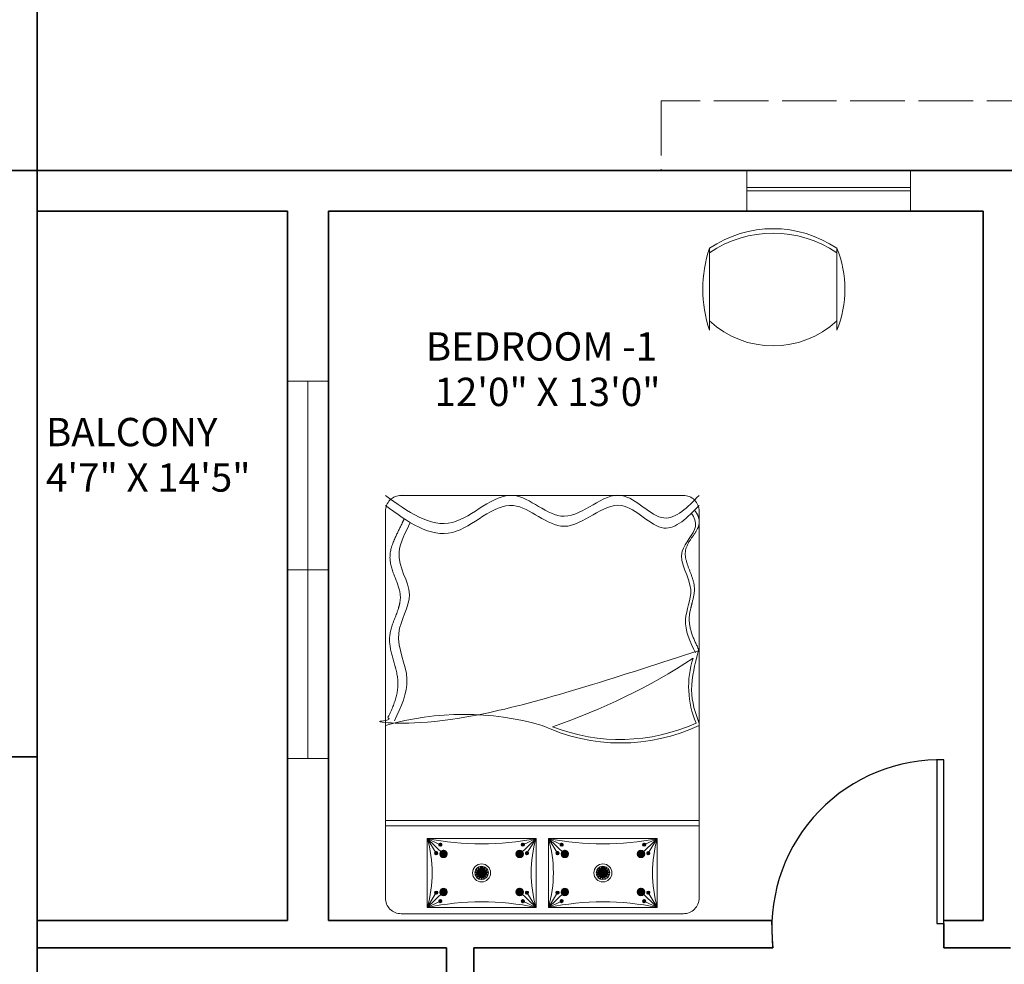
# Model space of a CAD drawing. Units: inches. Extents: x -61 to 1599, y -1316 to 257.
# Tile 166 of 204: x 998 to 1214, y -787 to -579. Entities that reach past the tile are written whole.
import ezdxf

# ---------------------------------------------------------------- set-up
doc = ezdxf.new("R2010")
doc.units = ezdxf.units.IN
doc.header["$MEASUREMENT"] = 0
doc.linetypes.add('ACAD_ISO02W100', pattern=[15, 12, -3])
for name, color, linetype, lineweight in [('A-AREA-IDEN', 1, 'Continuous', 18), ('A-FLOR-OVHD', 203, 'ACAD_ISO02W100', 13), ('A-WALL-JAMB', 4, 'ACAD_ISO02W100', 25), ('DOORS', 2, 'Continuous', 25), ('FURNITURE', 83, 'Continuous', 18), ('WALLS', 4, 'Continuous', 35), ('WINDOWS', 220, 'Continuous', 18)]:
    doc.layers.add(name, color=color, linetype=linetype, lineweight=lineweight)
doc.layers.add('LT', color=8, linetype='Continuous')
doc.styles.get("Standard").update_dxf_attribs({"font": 'arial.ttf'})

# ---------------------------------------------------------------- blocks, each defined once
blk = doc.blocks.new('DOOR-SWING-36')
blk.add_line((0, 0), (0, -5.4))
blk.add_lwpolyline([(0, 0), (0, 36), (-1.57, 36), (-1.57, 0)], close=True)
blk.add_arc((-0.74, -1.08), 37.09, 91.2913, 186.6905)
blk = doc.blocks.new('WIN-36IN')
for p, q in [((0, 4.5), (0, 9)), ((0, 9), (0, 0)), ((36, 9), (36, 0)), ((0, 5.26), (36, 5.26)), ((0, 4.5), (36, 4.5)), ((0, 4.5), (36, 4.5))]:
    blk.add_line(p, q)
blk = doc.blocks.new('WIN-83IN')
for p, q in [((0, 82.94), (9, 82.94)), ((0, 0), (9, 0))]:
    blk.add_line(p, q)
for points in [[(9, 82.94), (4.5, 82.94), (4.5, 41.47), (9, 41.47)], [(4.5, 41.47), (0, 41.47), (0, 0), (4.5, 0)]]:
    blk.add_lwpolyline(points, close=True)
blk = doc.blocks.new('BEDROOM-CHAIR')
for p, q in [((1.45, 3.47), (1.45, 21.47)), ((29.49, 3.47), (29.49, 21.47))]:
    blk.add_line(p, q)
for centre, radius, start, end in [((15.47, 0.83), 24.95, 55.8098, 124.1902), ((15.47, -0.17), 24.95, 55.8098, 124.1902), ((28.58, 12.47), 28.58, 161.6455, 198.3545), ((7.26, 12.47), 23.99, 337.9646, 22.0354), ((15.47, 20.69), 20.68, 227.332, 312.668)]:
    blk.add_arc(centre, radius, start, end)
blk = doc.blocks.new('*U15')
at = {"layer": 'LT'}
blk.add_line((0, 0.18), (0, -0.18), dxfattribs=at)
for centre, start, end in [((0.51, 0), 160.9983, 199.0017), ((-0.51, 0), 340.9983, 19.0017)]:
    blk.add_arc(centre, 0.539, start, end, dxfattribs=at)
blk = doc.blocks.new('*U16')
at = {"layer": 'LT', "transparency": 16777216}
for p, rotation in [((-66.65, -18.83), 96), ((-66.64, -18.76), 72), ((-66.63, -18.9), 120), ((-66.61, -18.69), 48.00000000000001), ((-66.58, -18.95), 144), ((-66.55, -18.65), 24), ((-66.51, -18.98), 168.0000000000001), ((-66.4, -18.65), 336.0000000000001), ((-66.37, -18.95), 216), ((-66.44, -18.98), 192), ((-66.34, -18.69), 312), ((-66.32, -18.9), 240), ((-66.31, -18.76), 288.0000000000001), ((-66.3, -18.83), 264)]:
    blk.add_blockref('*U15', p, dxfattribs=dict(at, rotation=rotation))
blk.add_blockref('*U15', (-66.48, -18.63), dxfattribs=at)
blk = doc.blocks.new('*U45')
at = {"layer": 'LT'}
blk.add_line((0, 0.18), (0, -0.18), dxfattribs=at)
for centre, start, end in [((0.51, 0), 160.9983, 199.0017), ((-0.51, 0), 340.9983, 19.0017)]:
    blk.add_arc(centre, 0.539, start, end, dxfattribs=at)
blk = doc.blocks.new('*U46')
at = {"layer": 'LT', "transparency": 16777216}
for p, rotation in [((-66.65, -18.83), 96), ((-66.64, -18.76), 72), ((-66.63, -18.9), 120), ((-66.61, -18.69), 48.00000000000001), ((-66.58, -18.95), 144), ((-66.55, -18.65), 24), ((-66.51, -18.98), 168.0000000000001), ((-66.4, -18.65), 336.0000000000001), ((-66.37, -18.95), 216), ((-66.44, -18.98), 192), ((-66.34, -18.69), 312), ((-66.32, -18.9), 240), ((-66.31, -18.76), 288.0000000000001), ((-66.3, -18.83), 264)]:
    blk.add_blockref('*U45', p, dxfattribs=dict(at, rotation=rotation))
blk.add_blockref('*U45', (-66.48, -18.63), dxfattribs=at)
blk = doc.blocks.new('*U9')
at = {"layer": 'LT'}
blk.add_line((0, 0.18), (0, -0.18), dxfattribs=at)
for centre, start, end in [((0.51, 0), 160.9983, 199.0017), ((-0.51, 0), 340.9983, 19.0017)]:
    blk.add_arc(centre, 0.539, start, end, dxfattribs=at)
blk = doc.blocks.new('*U10')
at = {"layer": 'LT', "transparency": 16777216}
for p, rotation in [((-66.65, -18.83), 96), ((-66.64, -18.76), 72), ((-66.63, -18.9), 120), ((-66.61, -18.69), 48.00000000000001), ((-66.58, -18.95), 144), ((-66.55, -18.65), 24), ((-66.51, -18.98), 168.0000000000001), ((-66.4, -18.65), 336.0000000000001), ((-66.37, -18.95), 216), ((-66.44, -18.98), 192), ((-66.34, -18.69), 312), ((-66.32, -18.9), 240), ((-66.31, -18.76), 288.0000000000001), ((-66.3, -18.83), 264)]:
    blk.add_blockref('*U9', p, dxfattribs=dict(at, rotation=rotation))
blk.add_blockref('*U9', (-66.48, -18.63), dxfattribs=at)
blk = doc.blocks.new('*U39')
at = {"layer": 'LT'}
blk.add_line((0, 0.18), (0, -0.18), dxfattribs=at)
for centre, start, end in [((0.51, 0), 160.9983, 199.0017), ((-0.51, 0), 340.9983, 19.0017)]:
    blk.add_arc(centre, 0.539, start, end, dxfattribs=at)
blk = doc.blocks.new('*U40')
at = {"layer": 'LT', "transparency": 16777216}
for p, rotation in [((-66.65, -18.83), 96), ((-66.64, -18.76), 72), ((-66.63, -18.9), 120), ((-66.61, -18.69), 48.00000000000001), ((-66.58, -18.95), 144), ((-66.55, -18.65), 24), ((-66.51, -18.98), 168.0000000000001), ((-66.4, -18.65), 336.0000000000001), ((-66.37, -18.95), 216), ((-66.44, -18.98), 192), ((-66.34, -18.69), 312), ((-66.32, -18.9), 240), ((-66.31, -18.76), 288.0000000000001), ((-66.3, -18.83), 264)]:
    blk.add_blockref('*U39', p, dxfattribs=dict(at, rotation=rotation))
blk.add_blockref('*U39', (-66.48, -18.63), dxfattribs=at)
blk = doc.blocks.new('*U17')
at = {"layer": 'LT'}
blk.add_line((0, 0.41), (0, -0.41), dxfattribs=at)
for centre, start, end in [((1.2, 0), 160.9983, 199.0017), ((-1.2, 0), 340.9983, 19.0017)]:
    blk.add_arc(centre, 1.27, start, end, dxfattribs=at)
blk = doc.blocks.new('*U18')
at = {"layer": 'LT', "transparency": 16777216}
for p, rotation in [((-156.74, -44.28), 96), ((-156.73, -44.11), 72), ((-156.69, -44.44), 120), ((-156.64, -43.96), 48.00000000000001), ((-156.58, -44.57), 144), ((-156.5, -43.86), 24), ((-156.42, -44.64), 168), ((-156.17, -43.86), 336.0000000000001), ((-156.25, -44.64), 192), ((-156.09, -44.57), 216), ((-156.03, -43.96), 312), ((-155.98, -44.44), 240), ((-155.94, -44.11), 288.0000000000001), ((-155.92, -44.28), 264)]:
    blk.add_blockref('*U17', p, dxfattribs=dict(at, rotation=rotation))
blk.add_blockref('*U17', (-156.33, -43.82), dxfattribs=at)
blk = doc.blocks.new('*U33')
at = {"layer": 'LT'}
blk.add_line((0, 0.41), (0, -0.41), dxfattribs=at)
for centre, start, end in [((1.2, 0), 160.9983, 199.0017), ((-1.2, 0), 340.9983, 19.0017)]:
    blk.add_arc(centre, 1.27, start, end, dxfattribs=at)
blk = doc.blocks.new('*U34')
at = {"layer": 'LT', "transparency": 16777216}
for p, rotation in [((-156.74, -44.28), 96), ((-156.73, -44.11), 72), ((-156.69, -44.44), 120), ((-156.64, -43.96), 48.00000000000001), ((-156.58, -44.57), 144), ((-156.5, -43.86), 24), ((-156.42, -44.64), 168), ((-156.17, -43.86), 336.0000000000001), ((-156.25, -44.64), 192), ((-156.09, -44.57), 216), ((-156.03, -43.96), 312), ((-155.98, -44.44), 240), ((-155.94, -44.11), 288.0000000000001), ((-155.92, -44.28), 264)]:
    blk.add_blockref('*U33', p, dxfattribs=dict(at, rotation=rotation))
blk.add_blockref('*U33', (-156.33, -43.82), dxfattribs=at)
blk = doc.blocks.new('*U11')
at = {"layer": 'LT'}
blk.add_line((0, 0.74), (0, -0.74), dxfattribs=at)
for centre, start, end in [((2.15, 0), 160.9983, 199.0017), ((-2.15, 0), 340.9983, 19.0017)]:
    blk.add_arc(centre, 2.27, start, end, dxfattribs=at)
blk = doc.blocks.new('*U12')
at = {"layer": 'LT', "transparency": 16777216}
for p, rotation in [((-280.54, -78.62), 23.99999999999999), ((-279.94, -78.62), 336.0000000000001), ((-280.98, -79.37), 96), ((-280.94, -79.07), 72), ((-280.88, -79.67), 120), ((-280.79, -78.8), 48.00000000000001), ((-280.68, -79.89), 144), ((-280.4, -80.02), 168), ((-280.09, -80.02), 191.9999999999999), ((-279.81, -79.89), 216), ((-279.69, -78.8), 312), ((-279.6, -79.67), 240), ((-279.54, -79.07), 288.0000000000001), ((-279.51, -79.37), 264)]:
    blk.add_blockref('*U11', p, dxfattribs=dict(at, rotation=rotation))
blk.add_blockref('*U11', (-280.24, -78.56), dxfattribs=at)
blk = doc.blocks.new('*U28')
at = {"layer": 'LT'}
blk.add_line((0, 0.41), (0, -0.41), dxfattribs=at)
for centre, start, end in [((1.2, 0), 160.9983, 199.0017), ((-1.2, 0), 340.9983, 19.0017)]:
    blk.add_arc(centre, 1.27, start, end, dxfattribs=at)
blk = doc.blocks.new('*U44')
at = {"layer": 'LT', "transparency": 16777216}
for p, rotation in [((-156.74, -44.28), 96), ((-156.73, -44.11), 72), ((-156.69, -44.44), 120), ((-156.64, -43.96), 48.00000000000001), ((-156.58, -44.57), 144), ((-156.5, -43.86), 24), ((-156.42, -44.64), 168), ((-156.17, -43.86), 336.0000000000001), ((-156.25, -44.64), 192), ((-156.09, -44.57), 216), ((-156.03, -43.96), 312), ((-155.98, -44.44), 240), ((-155.94, -44.11), 288.0000000000001), ((-155.92, -44.28), 264)]:
    blk.add_blockref('*U28', p, dxfattribs=dict(at, rotation=rotation))
blk.add_blockref('*U28', (-156.33, -43.82), dxfattribs=at)
blk = doc.blocks.new('*U13')
at = {"layer": 'LT'}
blk.add_line((0, 0.41), (0, -0.41), dxfattribs=at)
for centre, start, end in [((1.2, 0), 160.9983, 199.0017), ((-1.2, 0), 340.9983, 19.0017)]:
    blk.add_arc(centre, 1.27, start, end, dxfattribs=at)
blk = doc.blocks.new('*U14')
at = {"layer": 'LT', "transparency": 16777216}
for p, rotation in [((-156.74, -44.28), 96), ((-156.73, -44.11), 72), ((-156.69, -44.44), 120), ((-156.64, -43.96), 48.00000000000001), ((-156.58, -44.57), 144), ((-156.5, -43.86), 24), ((-156.42, -44.64), 168), ((-156.17, -43.86), 336.0000000000001), ((-156.25, -44.64), 192), ((-156.09, -44.57), 216), ((-156.03, -43.96), 312), ((-155.98, -44.44), 240), ((-155.94, -44.11), 288.0000000000001), ((-155.92, -44.28), 264)]:
    blk.add_blockref('*U13', p, dxfattribs=dict(at, rotation=rotation))
blk.add_blockref('*U13', (-156.33, -43.82), dxfattribs=at)
blk = doc.blocks.new('*U19')
at = {"layer": 'LT'}
blk.add_line((0, 0.18), (0, -0.18), dxfattribs=at)
for centre, start, end in [((0.51, 0), 160.9983, 199.0017), ((-0.51, 0), 340.9983, 19.0017)]:
    blk.add_arc(centre, 0.539, start, end, dxfattribs=at)
blk = doc.blocks.new('*U6')
at = {"layer": 'LT', "transparency": 16777216}
for p, rotation in [((-66.65, -18.83), 96), ((-66.64, -18.76), 72), ((-66.63, -18.9), 120), ((-66.61, -18.69), 48.00000000000001), ((-66.58, -18.95), 144), ((-66.55, -18.65), 24), ((-66.51, -18.98), 168.0000000000001), ((-66.4, -18.65), 336.0000000000001), ((-66.37, -18.95), 216), ((-66.44, -18.98), 192), ((-66.34, -18.69), 312), ((-66.32, -18.9), 240), ((-66.31, -18.76), 288.0000000000001), ((-66.3, -18.83), 264)]:
    blk.add_blockref('*U19', p, dxfattribs=dict(at, rotation=rotation))
blk.add_blockref('*U19', (-66.48, -18.63), dxfattribs=at)
blk = doc.blocks.new('*U35')
at = {"layer": 'LT'}
blk.add_line((0, 0.18), (0, -0.18), dxfattribs=at)
for centre, start, end in [((0.51, 0), 160.9983, 199.0017), ((-0.51, 0), 340.9983, 19.0017)]:
    blk.add_arc(centre, 0.539, start, end, dxfattribs=at)
blk = doc.blocks.new('*U36')
at = {"layer": 'LT', "transparency": 16777216}
for p, rotation in [((-66.65, -18.83), 96), ((-66.64, -18.76), 72), ((-66.63, -18.9), 120), ((-66.61, -18.69), 48.00000000000001), ((-66.58, -18.95), 144), ((-66.55, -18.65), 24), ((-66.51, -18.98), 168.0000000000001), ((-66.4, -18.65), 336.0000000000001), ((-66.37, -18.95), 216), ((-66.44, -18.98), 192), ((-66.34, -18.69), 312), ((-66.32, -18.9), 240), ((-66.31, -18.76), 288.0000000000001), ((-66.3, -18.83), 264)]:
    blk.add_blockref('*U35', p, dxfattribs=dict(at, rotation=rotation))
blk.add_blockref('*U35', (-66.48, -18.63), dxfattribs=at)
blk = doc.blocks.new('*U7')
at = {"layer": 'LT'}
blk.add_line((0, 0.18), (0, -0.18), dxfattribs=at)
for centre, start, end in [((0.51, 0), 160.9983, 199.0017), ((-0.51, 0), 340.9983, 19.0017)]:
    blk.add_arc(centre, 0.539, start, end, dxfattribs=at)
blk = doc.blocks.new('*U8')
at = {"layer": 'LT', "transparency": 16777216}
for p, rotation in [((-66.65, -18.83), 96), ((-66.64, -18.76), 72), ((-66.63, -18.9), 120), ((-66.61, -18.69), 48.00000000000001), ((-66.58, -18.95), 144), ((-66.55, -18.65), 24), ((-66.51, -18.98), 168.0000000000001), ((-66.4, -18.65), 336.0000000000001), ((-66.37, -18.95), 216), ((-66.44, -18.98), 192), ((-66.34, -18.69), 312), ((-66.32, -18.9), 240), ((-66.31, -18.76), 288.0000000000001), ((-66.3, -18.83), 264)]:
    blk.add_blockref('*U7', p, dxfattribs=dict(at, rotation=rotation))
blk.add_blockref('*U7', (-66.48, -18.63), dxfattribs=at)
blk = doc.blocks.new('*U37')
at = {"layer": 'LT'}
blk.add_line((0, 0.18), (0, -0.18), dxfattribs=at)
for centre, start, end in [((0.51, 0), 160.9983, 199.0017), ((-0.51, 0), 340.9983, 19.0017)]:
    blk.add_arc(centre, 0.539, start, end, dxfattribs=at)
blk = doc.blocks.new('*U38')
at = {"layer": 'LT', "transparency": 16777216}
for p, rotation in [((-66.65, -18.83), 96), ((-66.64, -18.76), 72), ((-66.63, -18.9), 120), ((-66.61, -18.69), 48.00000000000001), ((-66.58, -18.95), 144), ((-66.55, -18.65), 24), ((-66.51, -18.98), 168.0000000000001), ((-66.4, -18.65), 336.0000000000001), ((-66.37, -18.95), 216), ((-66.44, -18.98), 192), ((-66.34, -18.69), 312), ((-66.32, -18.9), 240), ((-66.31, -18.76), 288.0000000000001), ((-66.3, -18.83), 264)]:
    blk.add_blockref('*U37', p, dxfattribs=dict(at, rotation=rotation))
blk.add_blockref('*U37', (-66.48, -18.63), dxfattribs=at)
blk = doc.blocks.new('*U3')
at = {"layer": 'LT'}
blk.add_line((0, 0.18), (0, -0.18), dxfattribs=at)
for centre, start, end in [((0.51, 0), 160.9983, 199.0017), ((-0.51, 0), 340.9983, 19.0017)]:
    blk.add_arc(centre, 0.539, start, end, dxfattribs=at)
blk = doc.blocks.new('*U4')
at = {"layer": 'LT', "transparency": 16777216}
for p, rotation in [((-66.65, -18.83), 96), ((-66.64, -18.76), 72), ((-66.63, -18.9), 120), ((-66.61, -18.69), 48.00000000000001), ((-66.58, -18.95), 144), ((-66.55, -18.65), 24), ((-66.51, -18.98), 168.0000000000001), ((-66.4, -18.65), 336.0000000000001), ((-66.37, -18.95), 216), ((-66.44, -18.98), 192), ((-66.34, -18.69), 312), ((-66.32, -18.9), 240), ((-66.31, -18.76), 288.0000000000001), ((-66.3, -18.83), 264)]:
    blk.add_blockref('*U3', p, dxfattribs=dict(at, rotation=rotation))
blk.add_blockref('*U3', (-66.48, -18.63), dxfattribs=at)
blk = doc.blocks.new('*U20')
at = {"layer": 'LT'}
blk.add_line((0, 0.18), (0, -0.18), dxfattribs=at)
for centre, start, end in [((0.51, 0), 160.9983, 199.0017), ((-0.51, 0), 340.9983, 19.0017)]:
    blk.add_arc(centre, 0.539, start, end, dxfattribs=at)
blk = doc.blocks.new('*U21')
at = {"layer": 'LT', "transparency": 16777216}
for p, rotation in [((-66.65, -18.83), 96), ((-66.64, -18.76), 72), ((-66.63, -18.9), 120), ((-66.61, -18.69), 48.00000000000001), ((-66.58, -18.95), 144), ((-66.55, -18.65), 24), ((-66.51, -18.98), 168.0000000000001), ((-66.4, -18.65), 336.0000000000001), ((-66.37, -18.95), 216), ((-66.44, -18.98), 192), ((-66.34, -18.69), 312), ((-66.32, -18.9), 240), ((-66.31, -18.76), 288.0000000000001), ((-66.3, -18.83), 264)]:
    blk.add_blockref('*U20', p, dxfattribs=dict(at, rotation=rotation))
blk.add_blockref('*U20', (-66.48, -18.63), dxfattribs=at)
blk = doc.blocks.new('*U52')
at = {"layer": 'LT'}
blk.add_line((0, 0.18), (0, -0.18), dxfattribs=at)
for centre, start, end in [((0.51, 0), 160.9983, 199.0017), ((-0.51, 0), 340.9983, 19.0017)]:
    blk.add_arc(centre, 0.539, start, end, dxfattribs=at)
blk = doc.blocks.new('*U53')
at = {"layer": 'LT', "transparency": 16777216}
for p, rotation in [((-66.65, -18.83), 96), ((-66.64, -18.76), 72), ((-66.63, -18.9), 120), ((-66.61, -18.69), 48.00000000000001), ((-66.58, -18.95), 144), ((-66.55, -18.65), 24), ((-66.51, -18.98), 168.0000000000001), ((-66.4, -18.65), 336.0000000000001), ((-66.37, -18.95), 216), ((-66.44, -18.98), 192), ((-66.34, -18.69), 312), ((-66.32, -18.9), 240), ((-66.31, -18.76), 288.0000000000001), ((-66.3, -18.83), 264)]:
    blk.add_blockref('*U52', p, dxfattribs=dict(at, rotation=rotation))
blk.add_blockref('*U52', (-66.48, -18.63), dxfattribs=at)
blk = doc.blocks.new('*U29')
at = {"layer": 'LT'}
blk.add_line((0, 0.18), (0, -0.18), dxfattribs=at)
for centre, start, end in [((0.51, 0), 160.9983, 199.0017), ((-0.51, 0), 340.9983, 19.0017)]:
    blk.add_arc(centre, 0.539, start, end, dxfattribs=at)
blk = doc.blocks.new('*U30')
at = {"layer": 'LT', "transparency": 16777216}
for p, rotation in [((-66.65, -18.83), 96), ((-66.64, -18.76), 72), ((-66.63, -18.9), 120), ((-66.61, -18.69), 48.00000000000001), ((-66.58, -18.95), 144), ((-66.55, -18.65), 24), ((-66.51, -18.98), 168.0000000000001), ((-66.4, -18.65), 336.0000000000001), ((-66.37, -18.95), 216), ((-66.44, -18.98), 192), ((-66.34, -18.69), 312), ((-66.32, -18.9), 240), ((-66.31, -18.76), 288.0000000000001), ((-66.3, -18.83), 264)]:
    blk.add_blockref('*U29', p, dxfattribs=dict(at, rotation=rotation))
blk.add_blockref('*U29', (-66.48, -18.63), dxfattribs=at)
blk = doc.blocks.new('*U5')
at = {"layer": 'LT'}
blk.add_line((0, 0.41), (0, -0.41), dxfattribs=at)
for centre, start, end in [((1.2, 0), 160.9983, 199.0017), ((-1.2, 0), 340.9983, 19.0017)]:
    blk.add_arc(centre, 1.27, start, end, dxfattribs=at)
blk = doc.blocks.new('*U47')
at = {"layer": 'LT', "transparency": 16777216}
for p, rotation in [((-156.74, -44.28), 96), ((-156.73, -44.11), 72), ((-156.69, -44.44), 120), ((-156.64, -43.96), 48.00000000000001), ((-156.58, -44.57), 144), ((-156.5, -43.86), 24), ((-156.42, -44.64), 168), ((-156.17, -43.86), 336.0000000000001), ((-156.25, -44.64), 192), ((-156.09, -44.57), 216), ((-156.03, -43.96), 312), ((-155.98, -44.44), 240), ((-155.94, -44.11), 288.0000000000001), ((-155.92, -44.28), 264)]:
    blk.add_blockref('*U5', p, dxfattribs=dict(at, rotation=rotation))
blk.add_blockref('*U5', (-156.33, -43.82), dxfattribs=at)
blk = doc.blocks.new('*U22')
at = {"layer": 'LT'}
blk.add_line((0, 0.41), (0, -0.41), dxfattribs=at)
for centre, start, end in [((1.2, 0), 160.9983, 199.0017), ((-1.2, 0), 340.9983, 19.0017)]:
    blk.add_arc(centre, 1.27, start, end, dxfattribs=at)
blk = doc.blocks.new('*U23')
at = {"layer": 'LT', "transparency": 16777216}
for p, rotation in [((-156.74, -44.28), 96), ((-156.73, -44.11), 72), ((-156.69, -44.44), 120), ((-156.64, -43.96), 48.00000000000001), ((-156.58, -44.57), 144), ((-156.5, -43.86), 24), ((-156.42, -44.64), 168), ((-156.17, -43.86), 336.0000000000001), ((-156.25, -44.64), 192), ((-156.09, -44.57), 216), ((-156.03, -43.96), 312), ((-155.98, -44.44), 240), ((-155.94, -44.11), 288.0000000000001), ((-155.92, -44.28), 264)]:
    blk.add_blockref('*U22', p, dxfattribs=dict(at, rotation=rotation))
blk.add_blockref('*U22', (-156.33, -43.82), dxfattribs=at)
blk = doc.blocks.new('*U54')
at = {"layer": 'LT'}
blk.add_line((0, 0.74), (0, -0.74), dxfattribs=at)
for centre, start, end in [((2.15, 0), 160.9983, 199.0017), ((-2.15, 0), 340.9983, 19.0017)]:
    blk.add_arc(centre, 2.27, start, end, dxfattribs=at)
blk = doc.blocks.new('*U41')
at = {"layer": 'LT', "transparency": 16777216}
for p, rotation in [((-280.54, -78.62), 23.99999999999999), ((-279.94, -78.62), 336.0000000000001), ((-280.98, -79.37), 96), ((-280.94, -79.07), 72), ((-280.88, -79.67), 120), ((-280.79, -78.8), 48.00000000000001), ((-280.68, -79.89), 144), ((-280.4, -80.02), 168), ((-280.09, -80.02), 191.9999999999999), ((-279.81, -79.89), 216), ((-279.69, -78.8), 312), ((-279.6, -79.67), 240), ((-279.54, -79.07), 288.0000000000001), ((-279.51, -79.37), 264)]:
    blk.add_blockref('*U54', p, dxfattribs=dict(at, rotation=rotation))
blk.add_blockref('*U54', (-280.24, -78.56), dxfattribs=at)
blk = doc.blocks.new('*U42')
at = {"layer": 'LT'}
blk.add_line((0, 0.41), (0, -0.41), dxfattribs=at)
for centre, start, end in [((1.2, 0), 160.9983, 199.0017), ((-1.2, 0), 340.9983, 19.0017)]:
    blk.add_arc(centre, 1.27, start, end, dxfattribs=at)
blk = doc.blocks.new('*U43')
at = {"layer": 'LT', "transparency": 16777216}
for p, rotation in [((-156.74, -44.28), 96), ((-156.73, -44.11), 72), ((-156.69, -44.44), 120), ((-156.64, -43.96), 48.00000000000001), ((-156.58, -44.57), 144), ((-156.5, -43.86), 24), ((-156.42, -44.64), 168), ((-156.17, -43.86), 336.0000000000001), ((-156.25, -44.64), 192), ((-156.09, -44.57), 216), ((-156.03, -43.96), 312), ((-155.98, -44.44), 240), ((-155.94, -44.11), 288.0000000000001), ((-155.92, -44.28), 264)]:
    blk.add_blockref('*U42', p, dxfattribs=dict(at, rotation=rotation))
blk.add_blockref('*U42', (-156.33, -43.82), dxfattribs=at)
blk = doc.blocks.new('*U31')
at = {"layer": 'LT'}
blk.add_line((0, 0.41), (0, -0.41), dxfattribs=at)
for centre, start, end in [((1.2, 0), 160.9983, 199.0017), ((-1.2, 0), 340.9983, 19.0017)]:
    blk.add_arc(centre, 1.27, start, end, dxfattribs=at)
blk = doc.blocks.new('*U32')
at = {"layer": 'LT', "transparency": 16777216}
for p, rotation in [((-156.74, -44.28), 96), ((-156.73, -44.11), 72), ((-156.69, -44.44), 120), ((-156.64, -43.96), 48.00000000000001), ((-156.58, -44.57), 144), ((-156.5, -43.86), 24), ((-156.42, -44.64), 168), ((-156.17, -43.86), 336.0000000000001), ((-156.25, -44.64), 192), ((-156.09, -44.57), 216), ((-156.03, -43.96), 312), ((-155.98, -44.44), 240), ((-155.94, -44.11), 288.0000000000001), ((-155.92, -44.28), 264)]:
    blk.add_blockref('*U31', p, dxfattribs=dict(at, rotation=rotation))
blk.add_blockref('*U31', (-156.33, -43.82), dxfattribs=at)
blk = doc.blocks.new('*U48')
at = {"layer": 'LT'}
blk.add_line((0, 0.18), (0, -0.18), dxfattribs=at)
for centre, start, end in [((0.51, 0), 160.9983, 199.0017), ((-0.51, 0), 340.9983, 19.0017)]:
    blk.add_arc(centre, 0.539, start, end, dxfattribs=at)
blk = doc.blocks.new('*U49')
at = {"layer": 'LT', "transparency": 16777216}
for p, rotation in [((-66.65, -18.83), 96), ((-66.64, -18.76), 72), ((-66.63, -18.9), 120), ((-66.61, -18.69), 48.00000000000001), ((-66.58, -18.95), 144), ((-66.55, -18.65), 24), ((-66.51, -18.98), 168.0000000000001), ((-66.4, -18.65), 336.0000000000001), ((-66.37, -18.95), 216), ((-66.44, -18.98), 192), ((-66.34, -18.69), 312), ((-66.32, -18.9), 240), ((-66.31, -18.76), 288.0000000000001), ((-66.3, -18.83), 264)]:
    blk.add_blockref('*U48', p, dxfattribs=dict(at, rotation=rotation))
blk.add_blockref('*U48', (-66.48, -18.63), dxfattribs=at)
blk = doc.blocks.new('*U24')
at = {"layer": 'LT'}
blk.add_line((0, 0.18), (0, -0.18), dxfattribs=at)
for centre, start, end in [((0.51, 0), 160.9983, 199.0017), ((-0.51, 0), 340.9983, 19.0017)]:
    blk.add_arc(centre, 0.539, start, end, dxfattribs=at)
blk = doc.blocks.new('*U25')
at = {"layer": 'LT', "transparency": 16777216}
for p, rotation in [((-66.65, -18.83), 96), ((-66.64, -18.76), 72), ((-66.63, -18.9), 120), ((-66.61, -18.69), 48.00000000000001), ((-66.58, -18.95), 144), ((-66.55, -18.65), 24), ((-66.51, -18.98), 168.0000000000001), ((-66.4, -18.65), 336.0000000000001), ((-66.37, -18.95), 216), ((-66.44, -18.98), 192), ((-66.34, -18.69), 312), ((-66.32, -18.9), 240), ((-66.31, -18.76), 288.0000000000001), ((-66.3, -18.83), 264)]:
    blk.add_blockref('*U24', p, dxfattribs=dict(at, rotation=rotation))
blk.add_blockref('*U24', (-66.48, -18.63), dxfattribs=at)
blk = doc.blocks.new('*U50')
at = {"layer": 'LT'}
blk.add_line((0, 0.18), (0, -0.18), dxfattribs=at)
for centre, start, end in [((0.51, 0), 160.9983, 199.0017), ((-0.51, 0), 340.9983, 19.0017)]:
    blk.add_arc(centre, 0.539, start, end, dxfattribs=at)
blk = doc.blocks.new('*U51')
at = {"layer": 'LT', "transparency": 16777216}
for p, rotation in [((-66.65, -18.83), 96), ((-66.64, -18.76), 72), ((-66.63, -18.9), 120), ((-66.61, -18.69), 48.00000000000001), ((-66.58, -18.95), 144), ((-66.55, -18.65), 24), ((-66.51, -18.98), 168.0000000000001), ((-66.4, -18.65), 336.0000000000001), ((-66.37, -18.95), 216), ((-66.44, -18.98), 192), ((-66.34, -18.69), 312), ((-66.32, -18.9), 240), ((-66.31, -18.76), 288.0000000000001), ((-66.3, -18.83), 264)]:
    blk.add_blockref('*U50', p, dxfattribs=dict(at, rotation=rotation))
blk.add_blockref('*U50', (-66.48, -18.63), dxfattribs=at)
blk = doc.blocks.new('*U26')
at = {"layer": 'LT'}
blk.add_line((0, 0.18), (0, -0.18), dxfattribs=at)
for centre, start, end in [((0.51, 0), 160.9983, 199.0017), ((-0.51, 0), 340.9983, 19.0017)]:
    blk.add_arc(centre, 0.539, start, end, dxfattribs=at)
blk = doc.blocks.new('*U27')
at = {"layer": 'LT', "transparency": 16777216}
for p, rotation in [((-66.65, -18.83), 96), ((-66.64, -18.76), 72), ((-66.63, -18.9), 120), ((-66.61, -18.69), 48.00000000000001), ((-66.58, -18.95), 144), ((-66.55, -18.65), 24), ((-66.51, -18.98), 168.0000000000001), ((-66.4, -18.65), 336.0000000000001), ((-66.37, -18.95), 216), ((-66.44, -18.98), 192), ((-66.34, -18.69), 312), ((-66.32, -18.9), 240), ((-66.31, -18.76), 288.0000000000001), ((-66.3, -18.83), 264)]:
    blk.add_blockref('*U26', p, dxfattribs=dict(at, rotation=rotation))
blk.add_blockref('*U26', (-66.48, -18.63), dxfattribs=at)
blk = doc.blocks.new('BED-DOUBLE')
for p, q in [((1.27, 20.47), (70.26, 20.47)), ((1.27, 19.32), (70.26, 19.32)), ((10.47, 1.38), (10.47, 16.56)), ((34.39, 16.56), (10.47, 16.56)), ((10.47, 16.56), (13.35, 15.18)), ((10.47, 16.56), (14.04, 13.11)), ((10.47, 16.56), (12.45, 13.31)), ((13.35, 15.18), (13.35, 14.83)), ((34.39, 16.56), (30.82, 13.11)), ((34.39, 16.56), (31.51, 15.18)), ((31.51, 15.18), (31.51, 14.83)), ((34.39, 16.56), (32.4, 13.31)), ((37.15, 1.38), (37.15, 16.56)), ((61.06, 16.56), (37.15, 16.56)), ((37.15, 16.56), (40.03, 15.18)), ((37.15, 16.56), (40.71, 13.11)), ((37.15, 16.56), (39.13, 13.31)), ((40.03, 15.18), (40.03, 14.83)), ((61.06, 16.56), (57.5, 13.11)), ((61.06, 16.56), (58.18, 15.18)), ((58.18, 15.18), (58.18, 14.83)), ((61.06, 16.56), (59.08, 13.31)), ((12.45, 13.31), (12.45, 12.95)), ((14.05, 13.15), (14.05, 12.32)), ((30.81, 13.15), (30.81, 12.32)), ((32.4, 13.31), (32.4, 12.95)), ((39.13, 13.31), (39.13, 12.95)), ((40.73, 13.15), (40.73, 12.32)), ((57.48, 13.15), (57.48, 12.32)), ((59.08, 13.31), (59.08, 12.95)), ((22.43, 8.97), (22.43, 10.45)), ((49.11, 8.97), (49.11, 10.45)), ((10.47, 1.38), (14.04, 4.83)), ((10.47, 1.38), (12.45, 4.63)), ((12.45, 4.63), (12.45, 4.98)), ((14.05, 4.79), (14.05, 5.61)), ((30.81, 4.79), (30.81, 5.61)), ((34.39, 1.38), (30.82, 4.83)), ((32.4, 4.63), (32.4, 4.98)), ((34.39, 1.38), (32.4, 4.63)), ((37.15, 1.38), (40.71, 4.83)), ((37.15, 1.38), (39.13, 4.63)), ((39.13, 4.63), (39.13, 4.98)), ((40.73, 4.79), (40.73, 5.61)), ((57.48, 4.79), (57.48, 5.61)), ((61.06, 1.38), (57.5, 4.83)), ((59.08, 4.63), (59.08, 4.98)), ((61.06, 1.38), (59.08, 4.63)), ((10.47, 1.38), (13.35, 2.76)), ((13.35, 2.76), (13.35, 3.11)), ((31.51, 2.76), (31.51, 3.11)), ((34.39, 1.38), (31.51, 2.76)), ((37.15, 1.38), (40.03, 2.76)), ((40.03, 2.76), (40.03, 3.11)), ((58.18, 2.76), (58.18, 3.11)), ((61.06, 1.38), (58.18, 2.76)), ((34.39, 1.38), (34.39, 1.38)), ((61.06, 1.38), (61.06, 1.38))]:
    blk.add_line(p, q)
for points in [[(1.27, 88.54), (1.27, 3.45, 0.414214), (4.72, 0), (66.81, 0, 0.414214), (70.26, 3.45), (70.26, 88.54, 0.414214), (66.81, 91.99), (4.72, 91.99, 0.414214)], [(38.01, 41.13, 0.064396), (68.93, 56.18, 0.181766), (69.61, 41.92, -0.202767)], [(13.35, 15.18, 0.167358), (13.35, 14.83, 0.167358)], [(40.03, 15.18, 0.167358), (40.03, 14.83, 0.167358)], [(12.45, 13.31, 0.167358), (12.45, 12.95, 0.167358)], [(14.05, 13.15, 0.167358), (14.05, 12.32, 0.167358)], [(30.81, 12.32, 0.167358), (30.81, 13.15, 0.167358)], [(32.4, 12.95, 0.167358), (32.4, 13.31, 0.167358)], [(39.13, 13.31, 0.167358), (39.13, 12.95, 0.167358)], [(40.73, 13.15, 0.167358), (40.73, 12.32, 0.167358)], [(57.48, 12.32, 0.167358), (57.48, 13.15, 0.167358)], [(59.08, 12.95, 0.167358), (59.08, 13.31, 0.167358)], [(22.43, 8.97, 0.167358), (22.43, 10.45, 0.167358)], [(49.11, 8.97, 0.167358), (49.11, 10.45, 0.167358)], [(12.45, 4.98, 0.167358), (12.45, 4.63, 0.167358)], [(14.05, 5.61, 0.167358), (14.05, 4.79, 0.167358)], [(30.81, 4.79, 0.167358), (30.81, 5.61, 0.167358)], [(32.4, 4.63, 0.167358), (32.4, 4.98, 0.167358)], [(39.13, 4.98, 0.167358), (39.13, 4.63, 0.167358)], [(40.73, 5.61, 0.167358), (40.73, 4.79, 0.167358)], [(57.48, 4.79, 0.167358), (57.48, 5.61, 0.167358)], [(59.08, 4.63, 0.167358), (59.08, 4.98, 0.167358)], [(13.35, 3.11, 0.167358), (13.35, 2.76, 0.167358)], [(31.51, 2.76, 0.167358), (31.51, 3.11, 0.167358)], [(40.03, 3.11, 0.167358), (40.03, 2.76, 0.167358)], [(58.18, 2.76, 0.167358), (58.18, 3.11, 0.167358)]]:
    blk.add_lwpolyline(points, format="xyb", close=True)
blk.add_lwpolyline([(70.26, 41.39, -0.22309), (35.77, 41.39, 0.142156), (1.27, 41.39)], format="xyb")
for points in [[(34.39, 16.56), (34.39, 1.38), (10.47, 1.38), (10.47, 16.56), (34.39, 16.56), (34.39, 1.38), (10.47, 1.38)], [(61.06, 16.56), (61.06, 1.38), (37.15, 1.38)]]:
    blk.add_lwpolyline(points)
for centre, radius in [((13.35, 15.18), 0.351), ((31.51, 15.18), 0.351), ((40.03, 15.18), 0.351), ((58.18, 15.18), 0.351), ((12.45, 13.31), 0.351), ((14.05, 13.15), 0.825), ((30.81, 13.15), 0.825), ((32.4, 13.31), 0.351), ((39.13, 13.31), 0.351), ((40.73, 13.15), 0.825), ((57.48, 13.15), 0.825), ((59.08, 13.31), 0.351), ((22.43, 8.97), 1.98), ((49.11, 8.97), 1.98), ((22.43, 8.97), 1.48), ((49.11, 8.97), 1.48), ((12.45, 4.63), 0.351), ((14.05, 4.79), 0.825), ((30.81, 4.79), 0.825), ((32.4, 4.63), 0.351), ((39.13, 4.63), 0.351), ((40.73, 4.79), 0.825), ((57.48, 4.79), 0.825), ((59.08, 4.63), 0.351), ((13.35, 2.76), 0.351), ((31.51, 2.76), 0.351), ((40.03, 2.76), 0.351), ((58.18, 2.76), 0.351)]:
    blk.add_circle(centre, radius)
for centre, radius, start, end in [((-16, 8.97), 27.54, 344.0046, 15.9954), ((22.43, 74.54), 59.2, 258.3468, 281.6532), ((32.02, 15), 0.539, 160.9983, 199.0017), ((31, 15), 0.539, 340.9983, 19.0017), ((60.86, 8.97), 27.54, 164.0046, 195.9954), ((10.67, 8.97), 27.54, 344.0046, 15.9954), ((49.11, 74.54), 59.2, 258.3468, 281.6532), ((58.69, 15), 0.539, 160.9983, 199.0017), ((57.68, 15), 0.539, 340.9983, 19.0017), ((87.54, 8.97), 27.54, 164.0046, 195.9954), ((22.43, -56.6), 59.2, 78.3468, 101.6532), ((49.11, -56.6), 59.2, 78.3468, 101.6532)]:
    blk.add_arc(centre, radius, start, end)
for points, knots in [([(70.26, 91.99), (67.71, 89.38), (62.21, 83.76), (52.49, 96.72), (40.92, 82.74), (28.61, 96.74), (15.69, 81.53), (6.21, 88.41), (1.27, 91.99)], [0, 0, 0, 0, 9.176033, 19.753992, 33.150145, 45.209422, 59.881559, 75.764594, 75.764594, 75.764594, 75.764594]), ([(70.26, 89.76), (67.71, 87.16), (62.21, 81.54), (52.49, 94.5), (40.92, 80.52), (28.61, 94.52), (15.69, 79.31), (6.21, 86.19), (1.27, 89.76)], [0, 0, 0, 0, 9.176033, 19.753992, 33.150145, 45.209422, 59.881559, 75.764594, 75.764594, 75.764594, 75.764594]), ([(69.45, 57.36), (68.29, 59.79), (66.11, 64.34), (70.04, 71.91), (64.12, 79.11), (70.31, 84.4), (69.24, 87.09), (68.55, 88.05)], [0, 0, 0, 0, 6.649676, 12.451782, 19.973966, 25.324174, 28.349676, 28.349676, 28.349676, 28.349676]), ([(3.25, 42.44), (4.7, 45.45), (7.72, 51.72), (2.12, 61.25), (8.81, 70.52), (2.43, 77.93), (5.72, 83.91), (6.75, 86.04)], [0, 0, 0, 0, 8.27671, 17.241866, 24.903358, 33.244933, 38.427294, 38.427294, 38.427294, 38.427294])]:
    blk.add_open_spline(points, degree=3, knots=knots)
blk.add_open_spline([(5.01, 91.99), (4.99, 92.01), (4.96, 92.03), (4.94, 92.04)], degree=3)
for points, weights, knots in [([(70.26, 57.9), (59.86, 50.94), (48.6, 45.5), (36.68, 41.68), (36.46, 41.77), (36.25, 41.87), (36.03, 41.97), (24.6, 45.28), (12.69, 45.26), (1.27, 41.89), (2.72, 44.9), (5.74, 51.17), (0.14, 60.7), (6.83, 69.97), (0.11, 77.79), (4.35, 84.38), (5.4, 86.88)], [1, 0.993520320424, 0.993520320424, 1, 0.99997444972, 0.99997444972, 1, 0.973174868659, 0.973174868659, 1, 1, 1, 1, 1, 1, 1, 1], [0, 0, 0, 0, 0.279074, 0.279074, 0.279074, 0.296584, 0.296584, 0.296584, 0.865868, 0.865868, 0.865868, 9.142578, 18.107734, 25.769226, 34.110801, 40.441511, 40.441511, 40.441511, 40.441511]), ([(70.26, 41.83), (68.02, 47.03), (68.02, 52.7), (70.26, 57.9), (69.1, 60.33), (66.92, 64.87), (70.85, 72.44), (64.93, 79.65), (71.19, 84.99), (70.01, 87.73), (69.25, 88.74)], [1, 0.945466318698, 0.945466318698, 1, 1, 1, 1, 1, 1, 1, 1], [0, 0, 0, 0, 0.814571, 0.814571, 0.814571, 7.464247, 13.266353, 20.788537, 26.138745, 29.321895, 29.321895, 29.321895, 29.321895])]:
    blk.add_rational_spline(points, weights, degree=3, knots=knots)
for name, p in [('*U40', (79.83, 33.99)), ('*U30', (106.5, 33.99)), ('*U46', (78.93, 32.11)), ('*U34', (170.39, 57.38)), ('*U21', (105.61, 32.11)), ('*U23', (197.06, 57.38))]:
    blk.add_blockref(name, p)
at = {"extrusion": (0, 0, -1), "zscale": -1}
for name, p in [('*U36', (34.97, 33.99)), ('*U25', (8.29, 33.99)), ('*U14', (125.53, 57.38)), ('*U38', (34.07, 32.11)), ('*U32', (98.85, 57.38)), ('*U27', (7.39, 32.11))]:
    blk.add_blockref(name, p, dxfattribs=at)
at = {"rotation": 180}
for name, p in [('*U12', (-257.81, -70.33)), ('*U41', (-231.14, -70.33)), ('*U44', (-125.53, -39.45)), ('*U8', (-34.07, -14.18)), ('*U43', (-98.85, -39.45)), ('*U51', (-7.39, -14.18)), ('*U6', (-34.97, -16.05)), ('*U49', (-8.29, -16.05))]:
    blk.add_blockref(name, p, dxfattribs=at)
at = {"extrusion": (0, 0, -1), "zscale": -1, "rotation": 180}
for name, p in [('*U16', (-78.93, -14.18)), ('*U18', (-170.39, -39.45)), ('*U4', (-105.61, -14.18)), ('*U47', (-197.06, -39.45)), ('*U10', (-79.83, -16.05)), ('*U53', (-106.5, -16.05))]:
    blk.add_blockref(name, p, dxfattribs=at)

msp = doc.modelspace()

# ---------------------------------------------------------------- linework, layer by layer
at = {"layer": 'A-FLOR-OVHD'}
for p, q in [((1267.4807, -596.8766), (1138.8585, -596.8766)), ((1138.8585, -596.8766), (1138.8585, -612.169))]:
    msp.add_line(p, q, dxfattribs=at)
at = {"layer": 'A-WALL-JAMB'}
for p, q in [((1163.4756, -783.169), (1163.2611, -777.169)), ((1201.0506, -783.169), (1201.0506, -777.169))]:
    msp.add_line(p, q, dxfattribs=at)
at = {"layer": 'WALLS'}
for p, q in [((1001.7028, -432.3229), (1001.7028, -741.169)), ((1522.7028, -612.169), (992.7028, -612.169)), ((1001.7028, -621.169), (1001.7028, -777.169)), ((1001.7028, -621.169), (1056.7028, -621.169)), ((1056.7028, -621.169), (1056.7028, -777.169)), ((1065.7028, -621.169), (1065.7028, -777.169)), ((1065.7028, -621.169), (1209.7028, -621.169)), ((1209.7028, -621.169), (1209.7028, -777.169)), ((1001.7028, -741.169), (835.7028, -741.169)), ((1001.7028, -777.169), (1056.7028, -777.169)), ((1001.7028, -1202.169), (1001.7028, -777.169)), ((1065.7028, -777.169), (1163.2611, -777.169)), ((1201.0506, -777.169), (1209.7028, -777.169)), ((1001.7028, -783.169), (1091.7028, -783.169)), ((1091.7028, -939.169), (1091.7028, -783.169)), ((1097.7028, -783.169), (1163.4756, -783.169)), ((1097.7028, -939.169), (1097.7028, -783.169)), ((1201.0506, -783.169), (1215.7028, -783.169))]:
    msp.add_line(p, q, dxfattribs=at)

# ---------------------------------------------------------------- block references
at = {"layer": 'DOORS'}
msp.add_blockref('DOOR-SWING-36', (1201.0506, -777.769), dxfattribs=at)
at = {"layer": 'FURNITURE'}
for name, p in [('BEDROOM-CHAIR', (1148.039, -650.7671)), ('BED-DOUBLE', (1076.977, -775.6431))]:
    msp.add_blockref(name, p, dxfattribs=at)
at = {"layer": 'WINDOWS'}
for name, p in [('WIN-36IN', (1157.752, -621.1691)), ('WIN-83IN', (1056.703, -741.4811))]:
    msp.add_blockref(name, p, dxfattribs=at)

# ---------------------------------------------------------------- texts
at = {"layer": 'A-AREA-IDEN'}
for s, height, p in [('BEDROOM -1', 6.22364, (1087.1314, -653.9959)), (' 12\'0" X 13\'0"', 6.223643, (1087.1314, -663.9936)), ('BALCONY', 6.22364, (1003.5954, -672.8271)), ('4\'7" X 14\'5"', 6.223643, (1003.5954, -682.8249))]:
    msp.add_text(s, height=height, dxfattribs=at).set_placement(p)

doc.saveas('drawing.dxf')
